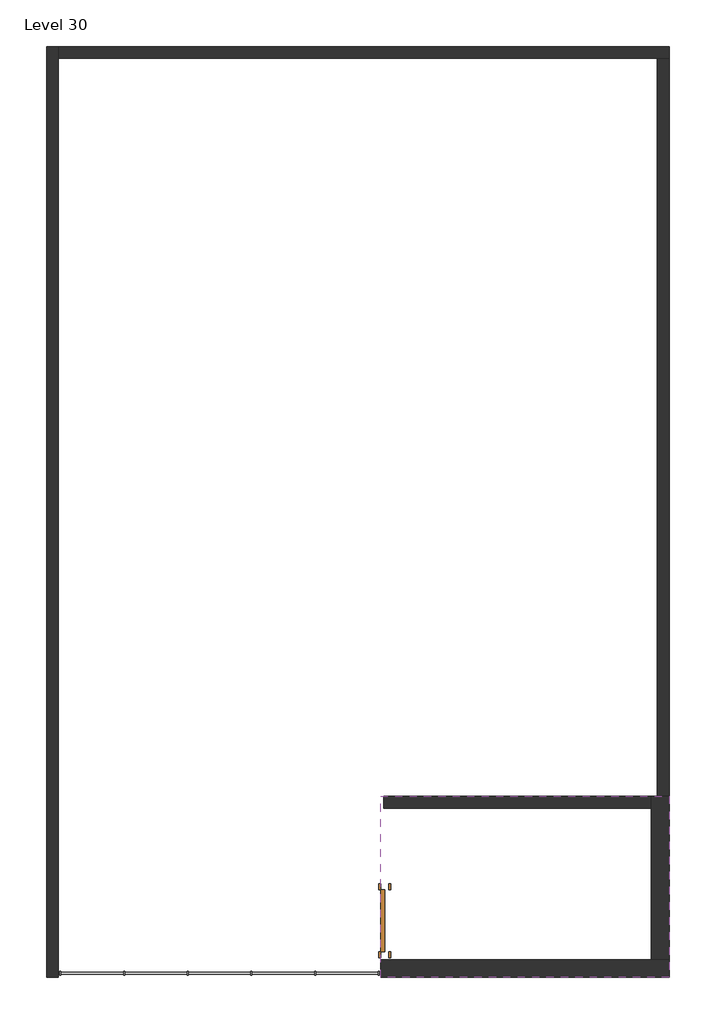
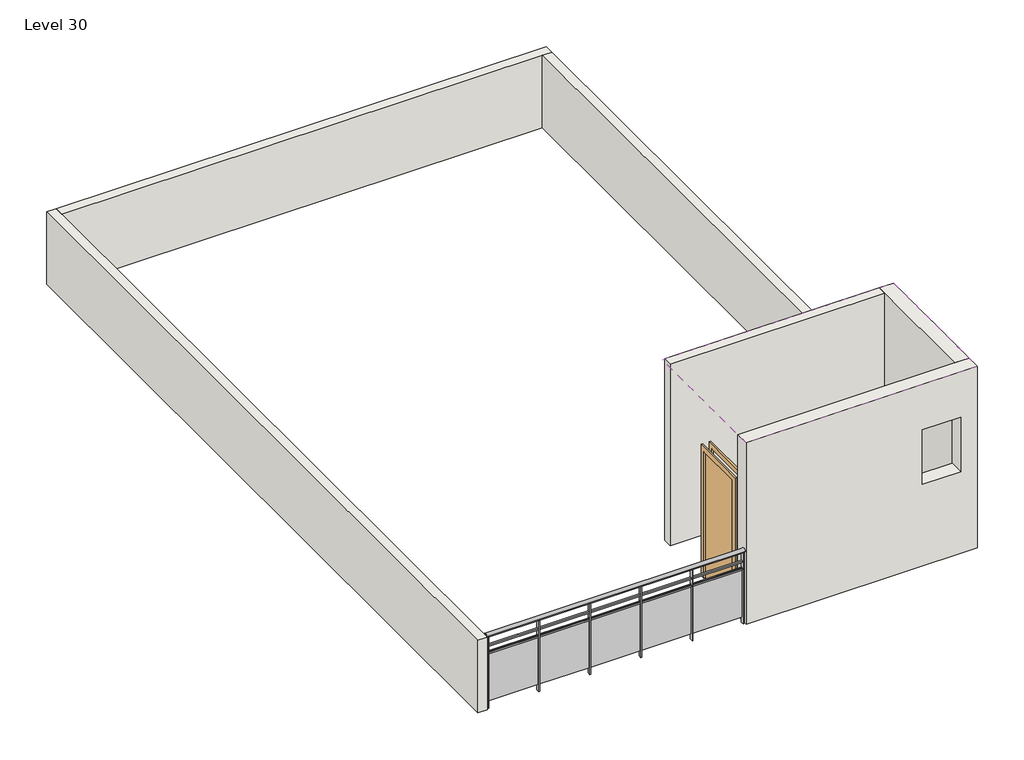
# One storey: 6 walls, 1 covering, 1 door, 1 railing.
"""IFC4 building model written with IfcOpenShell, lengths in millimetres."""

from ifc_helpers import new_model, si_unit, point, frame, origin, place, context, project, spatial, polyline, ellipse_curve, trimmed, outline, extrude, faceted_brep, transform, mapped, element, save
from ifc_brep_helpers import plane_surface, extruded_surface, advanced_brep
from components import door_c0900716

model = new_model("IFC4")

# Units and contexts
model_context = context("Model", 3, world=origin())
ifc_project = project(units=[si_unit("LENGTHUNIT", "METRE", prefix="MILLI")], contexts=[model_context])

# Site, building, storey
site = spatial("IfcSite", under=ifc_project)
building = spatial("IfcBuilding", under=site)
storey = spatial("IfcBuildingStorey", under=building, Name="Level 30", Elevation=28803.6)

# Covering
placement = place(None, origin())
element("IfcCovering", 1, ObjectType="2' x 4' ACT System", at=placement, inside=storey, context=model_context, shape_type="SweptSolid", body=[
    extrude(outline(polyline([(2041.0845537, -3670.5544725), (2041.0845537, -5981.9544725), (-1641.9154463, -5981.9544725), (-1641.9154463, -3670.5544725), (2041.0845537, -3670.5544725)])), frame((0.0, 0.0, 31851.6), z_axis=(0.0, 0.0, 1.0), x_axis=(1.0, 0.0, 0.0)), (0.0, 0.0, 1.0), 57.15),
])

# Door
door_shape = door_c0900716(model_context)
element("IfcDoor", 2, ObjectType="Single-Flush : 2'7\"", at=placement, inside=storey, context=model_context, shape_type="MappedRepresentation", body=[
    mapped(door_shape, transform((-1591.1154463, -5258.0544725, 28905.2), x_axis=(0.0, 1.0, 0.0), y_axis=(-1.0, 0.0, 0.0), z_axis=(0.0, 0.0, 1.0))),
])

# Railing
element("IfcRailing", 3, ObjectType="Glass Panel - Bottom Fill", at=placement, inside=storey, context=model_context, shape_type="SolidModel", body=[
    advanced_brep(
    [(-5756.7154463, -5893.0544725, 30022.8), (-5756.7154463, -5969.2544725, 30022.8), (-1641.9154463, -5893.0544725, 30022.8), (-1641.9154463, -5969.2544725, 30022.8)],
    [
        (0, 1, ellipse_curve(frame((-5756.7154463, -5931.1544725, 30022.8), z_axis=(-1.0, 0.0, 0.0), x_axis=(0.0, -1.0, 0.0)), 38.1, 28.575)),
        (1, 0, ellipse_curve(frame((-5756.7154463, -5931.1544725, 30022.8), z_axis=(-1.0, 0.0, 0.0), x_axis=(0.0, -1.0, 0.0)), 38.1, 28.575)),
        (2, 3, ellipse_curve(frame((-1641.9154463, -5931.1544725, 30022.8), z_axis=(1.0, 0.0, 0.0), x_axis=(0.0, -1.0, 0.0)), 38.1, 28.575)),
        (3, 2, ellipse_curve(frame((-1641.9154463, -5931.1544725, 30022.8), z_axis=(1.0, 0.0, 0.0), x_axis=(0.0, -1.0, 0.0)), 38.1, 28.575)),
        (0, 2),
        (3, 1),
    ],
    [
        plane_surface(frame((-5756.7154463, -5931.1544725, 30022.8), z_axis=(-1.0, 0.0, 0.0), x_axis=(0.0, 1.0, 0.0))),
        plane_surface(frame((-1641.9154463, -5931.1544725, 30022.8), z_axis=(1.0, 0.0, 0.0), x_axis=(0.0, 1.0, 0.0))),
        extruded_surface(trimmed(ellipse_curve(frame((-1641.9154463, -5931.1544725, 30022.8), z_axis=(-1.0, 0.0, 0.0), x_axis=(0.0, -1.0, 0.0)), 38.1, 28.575), [point((-1641.9154463, -5893.0544725, 30022.8))], [point((-1641.9154463, -5969.2544725, 30022.8))], True, "CARTESIAN"), (-4114.799999999999, 0.0, 0.0), 4114.799999999999),
        extruded_surface(trimmed(ellipse_curve(frame((-1641.9154463, -5931.1544725, 30022.8), z_axis=(-1.0, 0.0, 0.0), x_axis=(0.0, -1.0, 0.0)), 38.1, 28.575), [point((-1641.9154463, -5969.2544725, 30022.8))], [point((-1641.9154463, -5893.0544725, 30022.8))], True, "CARTESIAN"), (-4114.799999999999, 0.0, 0.0), 4114.799999999999),
    ],
    [
        (0, [[1, 2]]),
        (1, [[3, 4]]),
        (2, [[-1, 5, -4, 6]]),
        (3, [[-2, -6, -3, -5]]),
    ],
),
    extrude(outline(polyline([(-5756.7154463, -5943.8544725), (-5756.7154463, -5918.4544725), (-1641.9154463, -5918.4544725), (-1641.9154463, -5943.8544725), (-5756.7154463, -5943.8544725)])), frame((0.0, 0.0, 29832.3), z_axis=(0.0, 0.0, 1.0), x_axis=(1.0, 0.0, 0.0)), (0.0, 0.0, 1.0), 25.4),
    extrude(outline(polyline([(-5756.7154463, -5943.8544725), (-5756.7154463, -5918.4544725), (-1641.9154463, -5918.4544725), (-1641.9154463, -5943.8544725), (-5756.7154463, -5943.8544725)])), frame((0.0, 0.0, 29705.3), z_axis=(0.0, 0.0, 1.0), x_axis=(1.0, 0.0, 0.0)), (0.0, 0.0, 1.0), 25.4),
    extrude(outline(polyline([(-1673.6654463, -5956.5544725), (-1673.6654463, -5905.7544725), (-1660.9654463, -5905.7544725), (-1660.9654463, -5956.5544725), (-1673.6654463, -5956.5544725)])), frame((0.0, 0.0, 28803.6), z_axis=(0.0, 0.0, 1.0), x_axis=(1.0, 0.0, 0.0)), (0.0, 0.0, 1.0), 1190.625),
    extrude(outline(polyline([(-2480.1154463, -5924.6193155), (-1667.3154463, -5924.6193155), (-1667.3154463, -5930.9693155), (-2480.1154463, -5930.9693155), (-2480.1154463, -5924.6193155)])), frame((0.0, 0.0, 28905.2), z_axis=(0.0, 0.0, 1.0), x_axis=(1.0, 0.0, 0.0)), (0.0, 0.0, 1.0), 838.2),
    extrude(outline(polyline([(-2486.4654463, -5956.5544725), (-2486.4654463, -5905.7544725), (-2473.7654463, -5905.7544725), (-2473.7654463, -5956.5544725), (-2486.4654463, -5956.5544725)])), frame((0.0, 0.0, 28803.6), z_axis=(0.0, 0.0, 1.0), x_axis=(1.0, 0.0, 0.0)), (0.0, 0.0, 1.0), 1190.625),
    extrude(outline(polyline([(-3292.9154463, -5924.6193155), (-2480.1154463, -5924.6193155), (-2480.1154463, -5930.9693155), (-3292.9154463, -5930.9693155), (-3292.9154463, -5924.6193155)])), frame((0.0, 0.0, 28905.2), z_axis=(0.0, 0.0, 1.0), x_axis=(1.0, 0.0, 0.0)), (0.0, 0.0, 1.0), 838.2),
    extrude(outline(polyline([(-3299.2654463, -5956.5544725), (-3299.2654463, -5905.7544725), (-3286.5654463, -5905.7544725), (-3286.5654463, -5956.5544725), (-3299.2654463, -5956.5544725)])), frame((0.0, 0.0, 28803.6), z_axis=(0.0, 0.0, 1.0), x_axis=(1.0, 0.0, 0.0)), (0.0, 0.0, 1.0), 1190.625),
    extrude(outline(polyline([(-4105.7154463, -5924.6193155), (-3292.9154463, -5924.6193155), (-3292.9154463, -5930.9693155), (-4105.7154463, -5930.9693155), (-4105.7154463, -5924.6193155)])), frame((0.0, 0.0, 28905.2), z_axis=(0.0, 0.0, 1.0), x_axis=(1.0, 0.0, 0.0)), (0.0, 0.0, 1.0), 838.2),
    extrude(outline(polyline([(-4112.0654463, -5956.5544725), (-4112.0654463, -5905.7544725), (-4099.3654463, -5905.7544725), (-4099.3654463, -5956.5544725), (-4112.0654463, -5956.5544725)])), frame((0.0, 0.0, 28803.6), z_axis=(0.0, 0.0, 1.0), x_axis=(1.0, 0.0, 0.0)), (0.0, 0.0, 1.0), 1190.625),
    extrude(outline(polyline([(-4918.5154463, -5924.6193155), (-4105.7154463, -5924.6193155), (-4105.7154463, -5930.9693155), (-4918.5154463, -5930.9693155), (-4918.5154463, -5924.6193155)])), frame((0.0, 0.0, 28905.2), z_axis=(0.0, 0.0, 1.0), x_axis=(1.0, 0.0, 0.0)), (0.0, 0.0, 1.0), 838.2),
    extrude(outline(polyline([(-4924.8654463, -5956.5544725), (-4924.8654463, -5905.7544725), (-4912.1654463, -5905.7544725), (-4912.1654463, -5956.5544725), (-4924.8654463, -5956.5544725)])), frame((0.0, 0.0, 28803.6), z_axis=(0.0, 0.0, 1.0), x_axis=(1.0, 0.0, 0.0)), (0.0, 0.0, 1.0), 1190.625),
    extrude(outline(polyline([(-5731.3154463, -5924.6193155), (-4918.5154463, -5924.6193155), (-4918.5154463, -5930.9693155), (-5731.3154463, -5930.9693155), (-5731.3154463, -5924.6193155)])), frame((0.0, 0.0, 28905.2), z_axis=(0.0, 0.0, 1.0), x_axis=(1.0, 0.0, 0.0)), (0.0, 0.0, 1.0), 838.2),
    extrude(outline(polyline([(-5737.6654463, -5956.5544725), (-5737.6654463, -5905.7544725), (-5724.9654463, -5905.7544725), (-5724.9654463, -5956.5544725), (-5737.6654463, -5956.5544725)])), frame((0.0, 0.0, 28803.6), z_axis=(0.0, 0.0, 1.0), x_axis=(1.0, 0.0, 0.0)), (0.0, 0.0, 1.0), 1190.625),
    extrude(outline(polyline([(-1654.6154463, -5940.6794725), (-1654.6154463, -5921.6294725), (-1635.5654463, -5921.6294725), (-1635.5654463, -5940.6794725), (-1654.6154463, -5940.6794725)])), frame((0.0, 0.0, 28803.6), z_axis=(0.0, 0.0, 1.0), x_axis=(1.0, 0.0, 0.0)), (0.0, 0.0, 1.0), 1190.625),
    extrude(outline(polyline([(-5763.0654463, -5940.6794725), (-5763.0654463, -5921.6294725), (-5744.0154463, -5921.6294725), (-5744.0154463, -5940.6794725), (-5763.0654463, -5940.6794725)])), frame((0.0, 0.0, 28803.6), z_axis=(0.0, 0.0, 1.0), x_axis=(1.0, 0.0, 0.0)), (0.0, 0.0, 1.0), 1190.625),
])

# Walls
element("IfcWall", 4, ObjectType="Generic - 6\"", at=placement, inside=storey, context=model_context, shape_type="SweptSolid", body=[
    extrude(outline(polyline([(-1603.8154463, -3670.5544725), (1812.4845537, -3670.5544725), (1812.4845537, -3822.9544725), (-1603.8154463, -3822.9544725), (-1603.8154463, -3670.5544725)])), frame((0.0, 0.0, 28803.6), z_axis=(0.0, 0.0, 1.0), x_axis=(1.0, 0.0, 0.0)), (0.0, 0.0, 1.0), 3048.0),
])
element("IfcWall", 5, ObjectType="Generic - 6\"", at=placement, inside=storey, context=model_context, shape_type="Brep", body=[
    faceted_brep([(-5756.7154463, -5981.9544725, 28803.6), (-5756.7154463, 5754.4330275, 28803.6), (-5756.7154463, 5906.8330275, 28803.6), (-5756.7154463, 5906.8330275, 30022.8), (-5756.7154463, 5754.4330275, 30022.8), (-5756.7154463, -5981.9544725, 30022.8), (-5909.1154463, -5981.9544725, 28803.6), (-5909.1154463, -5981.9544725, 30022.8), (-5909.1154463, 5906.8330275, 30022.8), (-5909.1154463, 5906.8330275, 28803.6)], [[[0, 1, 2, 3, 4, 5]], [[6, 7, 8, 9]], [[2, 1, 0, 6, 9]], [[5, 4, 3, 8, 7]], [[0, 5, 7, 6]], [[3, 2, 9, 8]]]),
])
element("IfcWall", 6, ObjectType="Generic - 6\"", at=placement, inside=storey, context=model_context, shape_type="Brep", body=[
    faceted_brep([(-5756.7154463, 5754.4330275, 28803.6), (1888.6845537, 5754.4330275, 28803.6), (2041.0845537, 5754.4330275, 28803.6), (2041.0845537, 5754.4330275, 30022.8), (1888.6845537, 5754.4330275, 30022.8), (-5756.7154463, 5754.4330275, 30022.8), (-5756.7154463, 5906.8330275, 28803.6), (-5756.7154463, 5906.8330275, 30022.8), (2041.0845537, 5906.8330275, 30022.8), (2041.0845537, 5906.8330275, 28803.6)], [[[0, 1, 2, 3, 4, 5]], [[6, 7, 8, 9]], [[2, 1, 0, 6, 9]], [[5, 4, 3, 8, 7]], [[0, 5, 7, 6]], [[3, 2, 9, 8]]]),
])
element("IfcWall", 7, ObjectType="Generic - 6\"", at=placement, inside=storey, context=model_context, shape_type="SweptSolid", body=[
    extrude(outline(polyline([(1888.6845537, -3670.5544725), (1888.6845537, 5754.4330275), (2041.0845537, 5754.4330275), (2041.0845537, -3670.5544725), (1888.6845537, -3670.5544725)])), frame((0.0, 0.0, 28803.6), z_axis=(0.0, 0.0, 1.0), x_axis=(1.0, 0.0, 0.0)), (0.0, 0.0, 1.0), 1219.2),
])
element("IfcWall", 8, ObjectType="Generic - 9\"", at=placement, inside=storey, context=model_context, shape_type="Brep", body=[
    faceted_brep([(2041.0845537, -5753.3544725, 28803.6), (1812.4845537, -5753.3544725, 28803.6), (-1641.9154463, -5753.3544725, 28803.6), (-1641.9154463, -5753.3544725, 31851.6), (1812.4845537, -5753.3544725, 31851.6), (2041.0845537, -5753.3544725, 31851.6), (1164.7845537, -5753.3544725, 31089.6), (1164.7845537, -5753.3544725, 30175.2), (1774.3845537, -5753.3544725, 30175.2), (1774.3845537, -5753.3544725, 31089.6), (2041.0845537, -5981.9544725, 28803.6), (2041.0845537, -5981.9544725, 31851.6), (-1641.9154463, -5981.9544725, 31851.6), (-1641.9154463, -5981.9544725, 28803.6), (1164.7845537, -5981.9544725, 31089.6), (1774.3845537, -5981.9544725, 31089.6), (1774.3845537, -5981.9544725, 30175.2), (1164.7845537, -5981.9544725, 30175.2)], [[[0, 1, 2, 3, 4, 5], [6, 7, 8, 9]], [[10, 11, 12, 13], [14, 15, 16, 17]], [[2, 1, 0, 10, 13]], [[5, 4, 3, 12, 11]], [[0, 5, 11, 10]], [[3, 2, 13, 12]], [[7, 6, 14, 17]], [[8, 7, 17, 16]], [[9, 8, 16, 15]], [[6, 9, 15, 14]]]),
])
element("IfcWall", 9, ObjectType="Generic - 9\"", at=placement, inside=storey, context=model_context, shape_type="Brep", body=[
    faceted_brep([(2041.0845537, -5753.3544725, 28803.6), (2041.0845537, -3670.5544725, 28803.6), (2041.0845537, -3670.5544725, 30022.8), (2041.0845537, -3670.5544725, 31851.6), (2041.0845537, -5753.3544725, 31851.6), (1812.4845537, -5753.3544725, 28803.6), (1812.4845537, -5753.3544725, 31851.6), (1812.4845537, -3822.9544725, 31851.6), (1812.4845537, -3670.5544725, 31851.6), (1812.4845537, -3670.5544725, 28803.6), (1812.4845537, -3822.9544725, 28803.6), (1888.6845537, -3670.5544725, 28803.6)], [[[0, 1, 2, 3, 4]], [[5, 6, 7, 8, 9, 10]], [[1, 0, 5, 10, 9, 11]], [[4, 3, 8, 7, 6]], [[0, 4, 6, 5]], [[1, 11, 9, 8, 3, 2]]]),
])

save(model, "model.ifc")

# Revit data of these elements
# Type "2' x 4' ACT System"
#   Assembly Code = "C3030210"
#   built-in parameter 1002203 = 1 (stored number, unit not read)
#   built-in parameter 1002202 = 1 (stored number, unit not read)
#   Layers, outside or top first: 0' - 1 5/8" "Default" (function 1); 0' - 0 5/8" "Acoustic Ceiling Tile 24 x 48" (function 5)
# Type "Single-Flush : 2'7\""
#   Type Mark = "8"
#   Construction Type Id = "MDOOR"
#   Assembly Code = "C1020"
#   Analytic Construction = "Metal"
#   Thickness = 0' - 2"
#   Heat Transfer Coefficient (U) = 0.651978 BTU/(h·ft²·°F)
#   Height = 7' - 0"
#   Trim Projection Ext = 0' - 1"
#   Trim Projection Int = 0' - 1"
#   Trim Width = 0' - 3"
#   Width = 2' - 7"
#   Define Thermal Properties by = 1
#   Door Material = Door - Panel
#   Frame Material = Door - Frame
#   Visual Light Transmittance = 0
#   Solar Heat Gain Coefficient = 0
#   Function = (empty or 0)
#   Wall Closure = (empty or 0)
# Type "Glass Panel - Bottom Fill"
#   Assembly Code = "C2010400"
#   built-in parameter 1008612 = 0.0416667 (stored number, unit not read)
#   built-in parameter 1008611 = 0.0416667 (stored number, unit not read)
#   built-in parameter 1008609 = 0.333333 (stored number, unit not read)
#   built-in parameter 1008604 = 0.166667 (stored number, unit not read)
#   built-in parameter 1008603 = 0.166667 (stored number, unit not read)
#   Railing Height = 4' - 0"
#   built-in parameter 1008630 = 2
#   built-in parameter 1008610 = 2
#   built-in parameter 1008618 = Baluster - Square : 3/4"
# Type "Generic - 6\""
#   Assembly Code = "B2010"
#   Layers, outside or top first: 0' - 6" no material (function 1)
# Type "Generic - 9\""
#   Assembly Code = "B2010"
#   Layers, outside or top first: 0' - 9" no material (function 1)
# Element 1 (IfcCovering, "2' x 4' ACT System")
#   Height Offset From Level = 10' - 0"
#   Phase Created = New Construction
#   Materials on its faces: "Acoustic Ceiling Tile 24 x 48", "Default"
# Element 2 (IfcDoor, "Single-Flush : 2'7\"")
#   Phase Created = New Construction
#   Materials on its faces: "Door - Frame", "Door - Panel"
# Element 3 (IfcRailing, "Glass Panel - Bottom Fill")
#   Phase Created = New Construction
#   Materials on its faces: "Glass"
# Element 4 (IfcWall, "Generic - 6\"")
#   Top Offset = 0' - 0"
#   Base Offset = 0' - 0"
#   Unconnected Height = 10' - 0"
#   wall height = 10' - 0"
#   Phase Created = New Construction
#   Base Constraint = Level 30
#   Materials on its faces: "Default Wall"
# Elements 5, 6, 7 (IfcWall, "Generic - 6\"")
#   Top Offset = 0' - 0"
#   Base Offset = 0' - 0"
#   Unconnected Height = 4' - 0"
#   wall height = 4' - 0"
#   Phase Created = New Construction
#   Base Constraint = Level 30
#   Materials on its faces: "Default Wall"
# Elements 8, 9 (IfcWall, "Generic - 9\"")
#   Top Offset = 0' - 0"
#   Base Offset = 0' - 0"
#   Unconnected Height = 10' - 0"
#   wall height = 10' - 0"
#   Phase Created = New Construction
#   Base Constraint = Level 30
#   Materials on its faces: "Default Wall"
# Materials
#   "Default": colour RGB 127 127 127, transparency 0, Cost = 0
#   "Acoustic Ceiling Tile 24 x 48": class "Generic", colour RGB 229 229 229, transparency 0, Description = "Acoustic Ceiling Tile 24 x 48", Cost = 0
#   "Door - Panel": class "Wood", colour RGB 210 159 95, transparency 0, Cost = 0
#   "Door - Frame": colour RGB 118 70 51, transparency 0, Cost = 0
#   "Glass": class "Glass", colour RGB 0 128 192, transparency 0.75, Description = "Soda Lime Glass", Cost = 0
#   "Default Wall": colour RGB 128 128 128, transparency 0, Cost = 0
